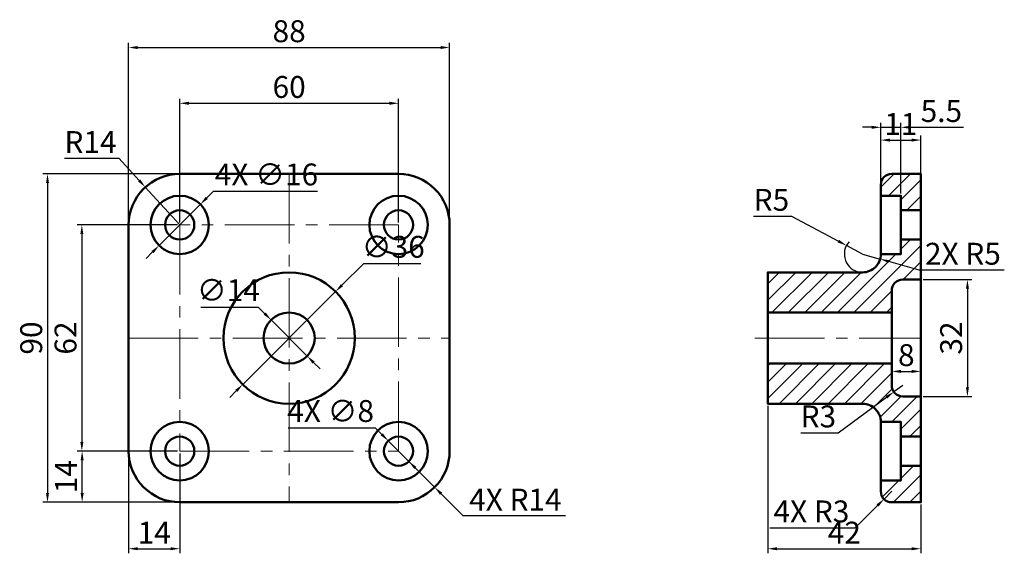
# Model space of a CAD drawing. Units: millimetres. Extents: x 7 to 277, y 39 to 185.
import ezdxf

# ---------------------------------------------------------------- set-up
doc = ezdxf.new("R2010")
doc.units = ezdxf.units.MM
doc.linetypes.add('CENTER2', pattern=[28.575, 19.05, -3.175, 3.175, -3.175])
for name, color, linetype, lineweight in [('M-CNTR', 4, 'CENTER2', 18), ('M-DIMS', 2, 'Continuous', 25), ('M-HATC', 8, 'Continuous', 18), ('M-OUTL', 7, 'Continuous', 50)]:
    doc.layers.add(name, color=color, linetype=linetype, lineweight=lineweight)
doc.styles.get("Standard").update_dxf_attribs({"font": 'arial.ttf'})
doc.dimstyles.new('ISO-25', dxfattribs={"dimtxt": 6, "dimasz": 2.5, "dimexe": 1.25, "dimexo": 0.625, "dimtad": 1, "dimtoh": 1, "dimdec": 0, "dimtxsty": 'Standard', "dimcen": 2.5, "dimadec": 0, "dimazin": 0, "dimtfac": 1, "dimtdec": 0, "dimtmove": 0, "dimatfit": 3, "dimfxl": 1, "dimarcsym": 0})

# ---------------------------------------------------------------- blocks, each defined once
blk = doc.blocks.new('*D1')
at = {"layer": 'Defpoints', "color": 0, "transparency": 16777216}
for p in [(233.41, 123.57), (237.82, 121.21)]:
    blk.add_point(p, dxfattribs=at)
at = {"layer": 'M-DIMS', "color": 0, "lineweight": -2, "transparency": 16777216}
for p, q in [((207.96, 131.63), (218.31, 131.63)), ((218.31, 131.63), (231.21, 124.75)), ((237.82, 121.21), (233.41, 123.57))]:
    blk.add_line(p, q, dxfattribs=at)
blk.add_arc((237.82, 121.21), 5, 137.5732, 262.838, dxfattribs=at)
at = {"layer": 'M-DIMS', "color": 0, "transparency": 16777216}
blk.add_solid([(231.4, 125.11), (231.01, 124.38), (233.41, 123.57)], dxfattribs=at)
at = {"layer": 'M-DIMS', "color": 0, "transparency": 16777216, "insert": (212.83, 135.31), "char_height": 6, "attachment_point": 5}
blk.add_mtext('R5', dxfattribs=at)
blk = doc.blocks.new('*D2')
at = {"layer": 'Defpoints', "color": 0, "transparency": 16777216}
for p in [(248.82, 85.21), (246.4, 83.44)]:
    blk.add_point(p, dxfattribs=at)
at = {"layer": 'M-DIMS', "color": 0, "lineweight": -2, "transparency": 16777216}
for p, q in [((248.82, 85.21), (246.4, 83.44)), ((231.16, 72.26), (244.39, 81.96)), ((220.86, 72.26), (231.16, 72.26))]:
    blk.add_line(p, q, dxfattribs=at)
at = {"layer": 'M-DIMS', "color": 0, "transparency": 16777216}
blk.add_solid([(244.14, 82.3), (244.63, 81.62), (246.4, 83.44)], dxfattribs=at)
at = {"layer": 'M-DIMS', "color": 0, "transparency": 16777216, "insert": (225.7, 75.95), "char_height": 6, "attachment_point": 5}
blk.add_mtext('R3', dxfattribs=at)
blk = doc.blocks.new('*D3')
at = {"layer": 'Defpoints', "color": 0, "transparency": 16777216}
for p in [(245.82, 91.21), (253.82, 91.21), (253.82, 89.06)]:
    blk.add_point(p, dxfattribs=at)
at = {"layer": 'M-DIMS', "color": 0, "lineweight": -2, "transparency": 16777216}
for p, q in [((245.82, 90.59), (245.82, 87.81)), ((253.82, 90.59), (253.82, 87.81)), ((248.32, 89.06), (251.32, 89.06))]:
    blk.add_line(p, q, dxfattribs=at)
at = {"layer": 'M-DIMS', "color": 0, "transparency": 16777216}
for points in [[(248.32, 89.48), (248.32, 88.65), (245.82, 89.06)], [(251.32, 89.48), (251.32, 88.65), (253.82, 89.06)]]:
    blk.add_solid(points, dxfattribs=at)
at = {"layer": 'M-DIMS', "color": 0, "transparency": 16777216, "insert": (249.82, 92.75), "char_height": 6, "attachment_point": 5}
blk.add_mtext('8', dxfattribs=at)
blk = doc.blocks.new('*D4')
at = {"layer": 'Defpoints', "color": 0, "transparency": 16777216}
for p in [(253.82, 152.47), (242.82, 137.21), (253.82, 137.21)]:
    blk.add_point(p, dxfattribs=at)
at = {"layer": 'M-DIMS', "color": 0, "lineweight": -2, "transparency": 16777216}
for p, q in [((242.82, 137.84), (242.82, 153.72)), ((245.32, 152.47), (251.32, 152.47)), ((253.82, 137.84), (253.82, 153.72))]:
    blk.add_line(p, q, dxfattribs=at)
at = {"layer": 'M-DIMS', "color": 0, "transparency": 16777216}
for points in [[(245.32, 152.88), (245.32, 152.05), (242.82, 152.47)], [(251.32, 152.88), (251.32, 152.05), (253.82, 152.47)]]:
    blk.add_solid(points, dxfattribs=at)
at = {"layer": 'M-DIMS', "color": 0, "transparency": 16777216, "insert": (248.32, 156.1), "char_height": 6, "attachment_point": 5}
blk.add_mtext('11', dxfattribs=at)
blk = doc.blocks.new('*D5')
at = {"layer": 'Defpoints', "color": 0, "transparency": 16777216}
for p in [(41.17, 139.56), (50.6, 129.21)]:
    blk.add_point(p, dxfattribs=at)
at = {"layer": 'M-DIMS', "color": 0, "lineweight": -2, "transparency": 16777216}
for p, q in [((18.98, 147.51), (33.91, 147.51)), ((33.91, 147.51), (39.48, 141.41)), ((50.6, 129.21), (41.17, 139.56))]:
    blk.add_line(p, q, dxfattribs=at)
at = {"layer": 'M-DIMS', "color": 0, "transparency": 16777216}
blk.add_solid([(39.79, 141.69), (39.17, 141.12), (41.17, 139.56)], dxfattribs=at)
at = {"layer": 'M-DIMS', "color": 0, "transparency": 16777216, "insert": (26.13, 151.15), "char_height": 6, "attachment_point": 5}
blk.add_mtext('R14', dxfattribs=at)
blk = doc.blocks.new('*D6')
at = {"layer": 'Defpoints', "color": 0, "transparency": 16777216}
for p in [(50.6, 129.21), (23.76, 67.21), (50.6, 67.21)]:
    blk.add_point(p, dxfattribs=at)
at = {"layer": 'M-DIMS', "color": 0, "lineweight": -2, "transparency": 16777216}
for p, q in [((49.97, 129.21), (22.51, 129.21)), ((23.76, 126.71), (23.76, 69.71)), ((49.97, 67.21), (22.51, 67.21))]:
    blk.add_line(p, q, dxfattribs=at)
at = {"layer": 'M-DIMS', "color": 0, "transparency": 16777216}
for points in [[(23.35, 126.71), (24.18, 126.71), (23.76, 129.21)], [(23.35, 69.71), (24.18, 69.71), (23.76, 67.21)]]:
    blk.add_solid(points, dxfattribs=at)
at = {"layer": 'M-DIMS', "color": 0, "transparency": 16777216, "insert": (20.07, 98.21), "char_height": 6, "attachment_point": 5, "rotation": 90}
blk.add_mtext('62', dxfattribs=at)
blk = doc.blocks.new('*D7')
at = {"layer": 'Defpoints', "color": 0, "transparency": 16777216}
for p in [(110.6, 162.55), (50.6, 129.21), (110.6, 129.21)]:
    blk.add_point(p, dxfattribs=at)
at = {"layer": 'M-DIMS', "color": 0, "lineweight": -2, "transparency": 16777216}
for p, q in [((50.6, 129.84), (50.6, 163.8)), ((53.1, 162.55), (108.1, 162.55)), ((110.6, 129.84), (110.6, 163.8))]:
    blk.add_line(p, q, dxfattribs=at)
at = {"layer": 'M-DIMS', "color": 0, "transparency": 16777216}
for points in [[(53.1, 162.97), (53.1, 162.13), (50.6, 162.55)], [(108.1, 162.97), (108.1, 162.13), (110.6, 162.55)]]:
    blk.add_solid(points, dxfattribs=at)
at = {"layer": 'M-DIMS', "color": 0, "transparency": 16777216, "insert": (80.6, 166.24), "char_height": 6, "attachment_point": 5}
blk.add_mtext('60', dxfattribs=at)
blk = doc.blocks.new('*D8')
at = {"layer": 'Defpoints', "color": 0, "transparency": 16777216}
for p in [(124.6, 177.83), (36.6, 109.01), (124.6, 109.01)]:
    blk.add_point(p, dxfattribs=at)
at = {"layer": 'M-DIMS', "color": 0, "lineweight": -2, "transparency": 16777216}
for p, q in [((36.6, 109.64), (36.6, 179.08)), ((124.6, 109.64), (124.6, 179.08)), ((39.1, 177.83), (122.1, 177.83))]:
    blk.add_line(p, q, dxfattribs=at)
at = {"layer": 'M-DIMS', "color": 0, "transparency": 16777216}
for points in [[(39.1, 178.25), (39.1, 177.41), (36.6, 177.83)], [(122.1, 178.25), (122.1, 177.41), (124.6, 177.83)]]:
    blk.add_solid(points, dxfattribs=at)
at = {"layer": 'M-DIMS', "color": 0, "transparency": 16777216, "insert": (80.6, 181.52), "char_height": 6, "attachment_point": 5}
blk.add_mtext('88', dxfattribs=at)
blk = doc.blocks.new('*D9')
at = {"layer": 'Defpoints', "color": 0, "transparency": 16777216}
for p in [(62.7, 143.21), (14.35, 53.21), (62.7, 53.21)]:
    blk.add_point(p, dxfattribs=at)
at = {"layer": 'M-DIMS', "color": 0, "lineweight": -2, "transparency": 16777216}
for p, q in [((62.07, 143.21), (13.1, 143.21)), ((14.35, 140.71), (14.35, 55.71)), ((62.07, 53.21), (13.1, 53.21))]:
    blk.add_line(p, q, dxfattribs=at)
at = {"layer": 'M-DIMS', "color": 0, "transparency": 16777216}
for points in [[(13.93, 140.71), (14.76, 140.71), (14.35, 143.21)], [(13.93, 55.71), (14.76, 55.71), (14.35, 53.21)]]:
    blk.add_solid(points, dxfattribs=at)
at = {"layer": 'M-DIMS', "color": 0, "transparency": 16777216, "insert": (10.66, 98.21), "char_height": 6, "attachment_point": 5, "rotation": 90}
blk.add_mtext('90', dxfattribs=at)
blk = doc.blocks.new('HOLE-CBORE-D8-D16')
for radius in [8, 4]:
    blk.add_circle((8, 8), radius)
blk = doc.blocks.new('*D11')
at = {"layer": 'Defpoints', "color": 0, "transparency": 16777216}
for p in [(211.82, 80.21), (253.82, 53.21), (253.82, 40.46)]:
    blk.add_point(p, dxfattribs=at)
at = {"layer": 'M-DIMS', "color": 0, "lineweight": -2, "transparency": 16777216}
for p, q in [((211.82, 79.59), (211.82, 39.21)), ((253.82, 52.59), (253.82, 39.21)), ((214.32, 40.46), (251.32, 40.46))]:
    blk.add_line(p, q, dxfattribs=at)
at = {"layer": 'M-DIMS', "color": 0, "transparency": 16777216}
for points in [[(214.32, 40.88), (214.32, 40.05), (211.82, 40.46)], [(251.32, 40.88), (251.32, 40.05), (253.82, 40.46)]]:
    blk.add_solid(points, dxfattribs=at)
at = {"layer": 'M-DIMS', "color": 0, "transparency": 16777216, "insert": (232.82, 44.1), "char_height": 6, "attachment_point": 5}
blk.add_mtext('42', dxfattribs=at)
blk = doc.blocks.new('*D12')
at = {"layer": 'Defpoints', "color": 0, "transparency": 16777216}
for p in [(253.82, 114.21), (253.82, 82.21), (266.57, 82.21)]:
    blk.add_point(p, dxfattribs=at)
at = {"layer": 'M-DIMS', "color": 0, "lineweight": -2, "transparency": 16777216}
for p, q in [((254.45, 114.21), (267.82, 114.21)), ((266.57, 111.71), (266.57, 84.71)), ((254.45, 82.21), (267.82, 82.21))]:
    blk.add_line(p, q, dxfattribs=at)
at = {"layer": 'M-DIMS', "color": 0, "transparency": 16777216}
for points in [[(266.16, 111.71), (266.99, 111.71), (266.57, 114.21)], [(266.16, 84.71), (266.99, 84.71), (266.57, 82.21)]]:
    blk.add_solid(points, dxfattribs=at)
at = {"layer": 'M-DIMS', "color": 0, "transparency": 16777216, "insert": (262.88, 98.21), "char_height": 6, "attachment_point": 5, "rotation": 90}
blk.add_mtext('32', dxfattribs=at)
blk = doc.blocks.new('*D13')
at = {"layer": 'Defpoints', "color": 0, "transparency": 16777216}
for p in [(248.32, 155.96), (242.82, 137.21), (248.32, 137.21)]:
    blk.add_point(p, dxfattribs=at)
at = {"layer": 'M-DIMS', "color": 0, "lineweight": -2, "transparency": 16777216}
for p, q in [((242.82, 137.84), (242.82, 157.21)), ((248.32, 137.84), (248.32, 157.21)), ((240.32, 155.96), (237.82, 155.96)), ((242.82, 155.96), (248.32, 155.96)), ((250.82, 155.96), (265.54, 155.96))]:
    blk.add_line(p, q, dxfattribs=at)
at = {"layer": 'M-DIMS', "color": 0, "transparency": 16777216}
for points in [[(240.32, 156.38), (240.32, 155.55), (242.82, 155.96)], [(250.82, 156.38), (250.82, 155.55), (248.32, 155.96)]]:
    blk.add_solid(points, dxfattribs=at)
at = {"layer": 'M-DIMS', "color": 0, "transparency": 16777216, "insert": (259.43, 159.64), "char_height": 6, "attachment_point": 5}
blk.add_mtext('5.5', dxfattribs=at)
blk = doc.blocks.new('*D14')
at = {"layer": 'Defpoints', "color": 0, "transparency": 16777216}
for p in [(36.6, 67.21), (50.6, 67.21), (50.6, 40.46)]:
    blk.add_point(p, dxfattribs=at)
at = {"layer": 'M-DIMS', "color": 0, "lineweight": -2, "transparency": 16777216}
for p, q in [((36.6, 66.59), (36.6, 39.21)), ((50.6, 66.59), (50.6, 39.21)), ((39.1, 40.46), (48.1, 40.46))]:
    blk.add_line(p, q, dxfattribs=at)
at = {"layer": 'M-DIMS', "color": 0, "transparency": 16777216}
for points in [[(39.1, 40.88), (39.1, 40.05), (36.6, 40.46)], [(48.1, 40.88), (48.1, 40.05), (50.6, 40.46)]]:
    blk.add_solid(points, dxfattribs=at)
at = {"layer": 'M-DIMS', "color": 0, "transparency": 16777216, "insert": (43.6, 44.1), "char_height": 6, "attachment_point": 5}
blk.add_mtext('14', dxfattribs=at)
blk = doc.blocks.new('*D15')
at = {"layer": 'Defpoints', "color": 0, "transparency": 16777216}
for p in [(23.85, 67.21), (50.6, 67.21), (50.6, 53.21)]:
    blk.add_point(p, dxfattribs=at)
at = {"layer": 'M-DIMS', "color": 0, "lineweight": -2, "transparency": 16777216}
for p, q in [((49.97, 67.21), (22.6, 67.21)), ((23.85, 55.71), (23.85, 64.71)), ((49.97, 53.21), (22.6, 53.21))]:
    blk.add_line(p, q, dxfattribs=at)
at = {"layer": 'M-DIMS', "color": 0, "transparency": 16777216}
for points in [[(23.43, 64.71), (24.26, 64.71), (23.85, 67.21)], [(23.43, 55.71), (24.26, 55.71), (23.85, 53.21)]]:
    blk.add_solid(points, dxfattribs=at)
at = {"layer": 'M-DIMS', "color": 0, "transparency": 16777216, "insert": (20.21, 60.21), "char_height": 6, "attachment_point": 5, "rotation": 90}
blk.add_mtext('14', dxfattribs=at)
blk = doc.blocks.new('*D16')
at = {"layer": 'Defpoints', "color": 0, "transparency": 16777216}
for p in [(110.6, 67.21), (120.5, 57.31)]:
    blk.add_point(p, dxfattribs=at)
at = {"layer": 'M-DIMS', "color": 0, "lineweight": -2, "transparency": 16777216}
for p, q in [((110.6, 67.21), (120.5, 57.31)), ((128.3, 49.52), (122.27, 55.55)), ((156.37, 49.52), (128.3, 49.52))]:
    blk.add_line(p, q, dxfattribs=at)
at = {"layer": 'M-DIMS', "color": 0, "transparency": 16777216}
blk.add_solid([(122.56, 55.84), (121.97, 55.25), (120.5, 57.31)], dxfattribs=at)
at = {"layer": 'M-DIMS', "color": 0, "transparency": 16777216, "insert": (142.64, 53.16), "char_height": 6, "attachment_point": 5}
blk.add_mtext('4X R14', dxfattribs=at)
blk = doc.blocks.new('*D17')
at = {"layer": 'Defpoints', "color": 0, "transparency": 16777216}
for p in [(56.26, 134.87), (44.94, 123.56)]:
    blk.add_point(p, dxfattribs=at)
at = {"layer": 'M-DIMS', "color": 0, "lineweight": -2, "transparency": 16777216}
for p, q in [((59.79, 138.41), (58.02, 136.64)), ((88.35, 138.41), (59.79, 138.41)), ((44.94, 123.56), (56.26, 134.87)), ((43.17, 121.79), (41.41, 120.02))]:
    blk.add_line(p, q, dxfattribs=at)
at = {"layer": 'M-DIMS', "color": 0, "transparency": 16777216}
for points in [[(57.73, 136.93), (58.32, 136.34), (56.26, 134.87)], [(42.88, 122.08), (43.47, 121.49), (44.94, 123.56)]]:
    blk.add_solid(points, dxfattribs=at)
at = {"layer": 'M-DIMS', "color": 0, "transparency": 16777216, "insert": (74.38, 142.26), "char_height": 6, "attachment_point": 5}
blk.add_mtext('4X ∅16', dxfattribs=at)
blk = doc.blocks.new('*D18')
at = {"layer": 'Defpoints', "color": 0, "transparency": 16777216}
for p in [(107.77, 70.04), (113.43, 64.38)]:
    blk.add_point(p, dxfattribs=at)
at = {"layer": 'M-DIMS', "color": 0, "lineweight": -2, "transparency": 16777216}
for p, q in [((80.32, 73.58), (104.23, 73.58)), ((104.23, 73.58), (106, 71.81)), ((113.43, 64.38), (107.77, 70.04)), ((115.19, 62.62), (116.96, 60.85))]:
    blk.add_line(p, q, dxfattribs=at)
at = {"layer": 'M-DIMS', "color": 0, "transparency": 16777216}
for points in [[(106.3, 72.1), (105.71, 71.52), (107.77, 70.04)], [(115.49, 62.91), (114.9, 62.32), (113.43, 64.38)]]:
    blk.add_solid(points, dxfattribs=at)
at = {"layer": 'M-DIMS', "color": 0, "transparency": 16777216, "insert": (91.97, 77.43), "char_height": 6, "attachment_point": 5}
blk.add_mtext('4X ∅8', dxfattribs=at)
blk = doc.blocks.new('*D19')
at = {"layer": 'Defpoints', "color": 0, "transparency": 16777216}
for p in [(93.33, 110.94), (67.87, 85.49)]:
    blk.add_point(p, dxfattribs=at)
at = {"layer": 'M-DIMS', "color": 0, "lineweight": -2, "transparency": 16777216}
for p, q in [((100.96, 118.58), (95.09, 112.71)), ((116.71, 118.58), (100.96, 118.58)), ((67.87, 85.49), (93.33, 110.94)), ((66.1, 83.72), (64.33, 81.95))]:
    blk.add_line(p, q, dxfattribs=at)
at = {"layer": 'M-DIMS', "color": 0, "transparency": 16777216}
for points in [[(94.8, 113), (95.39, 112.41), (93.33, 110.94)], [(65.81, 84.01), (66.4, 83.42), (67.87, 85.49)]]:
    blk.add_solid(points, dxfattribs=at)
at = {"layer": 'M-DIMS', "color": 0, "transparency": 16777216, "insert": (109.15, 122.43), "char_height": 6, "attachment_point": 5}
blk.add_mtext('∅36', dxfattribs=at)
blk = doc.blocks.new('*D20')
at = {"layer": 'Defpoints', "color": 0, "transparency": 16777216}
for p in [(75.65, 103.16), (85.55, 93.26)]:
    blk.add_point(p, dxfattribs=at)
at = {"layer": 'M-DIMS', "color": 0, "lineweight": -2, "transparency": 16777216}
for p, q in [((56.39, 106.7), (72.11, 106.7)), ((72.11, 106.7), (73.88, 104.93)), ((85.55, 93.26), (75.65, 103.16)), ((87.32, 91.5), (89.08, 89.73))]:
    blk.add_line(p, q, dxfattribs=at)
at = {"layer": 'M-DIMS', "color": 0, "transparency": 16777216}
for points in [[(74.17, 105.23), (73.59, 104.64), (75.65, 103.16)], [(87.61, 91.79), (87.02, 91.2), (85.55, 93.26)]]:
    blk.add_solid(points, dxfattribs=at)
at = {"layer": 'M-DIMS', "color": 0, "transparency": 16777216, "insert": (63.94, 110.55), "char_height": 6, "attachment_point": 5}
blk.add_mtext('∅14', dxfattribs=at)
blk = doc.blocks.new('*D21')
at = {"layer": 'Defpoints', "color": 0, "transparency": 16777216}
for p in [(237.82, 121.21), (242.63, 119.86)]:
    blk.add_point(p, dxfattribs=at)
at = {"layer": 'M-DIMS', "color": 0, "lineweight": -2, "transparency": 16777216}
for p, q in [((237.82, 121.21), (242.63, 119.86)), ((253.35, 116.84), (245.04, 119.18)), ((276.69, 116.84), (253.35, 116.84))]:
    blk.add_line(p, q, dxfattribs=at)
at = {"layer": 'M-DIMS', "color": 0, "transparency": 16777216}
blk.add_solid([(245.15, 119.58), (244.93, 118.78), (242.63, 119.86)], dxfattribs=at)
at = {"layer": 'M-DIMS', "color": 0, "transparency": 16777216, "insert": (265.33, 120.53), "char_height": 6, "attachment_point": 5}
blk.add_mtext('2X R5', dxfattribs=at)
blk = doc.blocks.new('*D22')
at = {"layer": 'Defpoints', "color": 0, "transparency": 16777216}
for p in [(243.7, 54.09), (245.82, 56.21)]:
    blk.add_point(p, dxfattribs=at)
at = {"layer": 'M-DIMS', "color": 0, "lineweight": -2, "transparency": 16777216}
for p, q in [((245.82, 56.21), (243.7, 54.09)), ((235.83, 46.22), (241.93, 52.32)), ((212.39, 46.22), (235.83, 46.22))]:
    blk.add_line(p, q, dxfattribs=at)
at = {"layer": 'M-DIMS', "color": 0, "transparency": 16777216}
blk.add_solid([(241.64, 52.62), (242.23, 52.03), (243.7, 54.09)], dxfattribs=at)
at = {"layer": 'M-DIMS', "color": 0, "transparency": 16777216, "insert": (223.8, 49.91), "char_height": 6, "attachment_point": 5}
blk.add_mtext('4X R3', dxfattribs=at)

msp = doc.modelspace()

# ---------------------------------------------------------------- hatches: boundary and pattern name
at = {"layer": 'M-HATC'}
h = msp.add_hatch(dxfattribs=at)
h.set_pattern_fill('ANSI31', color=256)
h.paths.add_polyline_path([(253.82, 143.21), (245.82, 143.21, 0.414214), (242.82, 140.21), (242.82, 137.21), (248.32, 137.21), (248.32, 133.21), (253.82, 133.21)])
h.paths.add_polyline_path([(248.82, 114.21), (253.82, 114.21), (253.82, 125.21), (248.32, 125.21), (248.32, 121.21), (242.82, 121.21, -0.414214), (237.82, 116.21), (211.82, 116.21), (211.82, 105.21), (245.82, 105.21), (245.82, 111.21, -0.414214)])
h.paths.add_polyline_path([(245.82, 91.21), (211.82, 91.21), (211.82, 80.21), (237.82, 80.21, -0.414214), (242.82, 75.21), (248.32, 75.21), (248.32, 71.21), (253.82, 71.21), (253.82, 82.21), (248.82, 82.21, -0.414214), (245.82, 85.21)])
h.paths.add_polyline_path([(253.82, 63.21), (248.32, 63.21), (248.32, 59.21), (242.82, 59.21), (242.82, 56.21, 0.414214), (245.82, 53.21), (253.82, 53.21)])

# ---------------------------------------------------------------- linework, layer by layer
at = {"layer": 'M-CNTR'}
for p, q in [((80.6, 143.21), (80.6, 53.21)), ((36.6, 98.21), (124.6, 98.21)), ((208.32, 98.21), (253.82, 98.21))]:
    msp.add_line(p, q, dxfattribs=at)
msp.add_lwpolyline([(110.6, 67.21), (110.6, 129.21), (50.6, 129.21), (50.6, 67.21)], close=True, dxfattribs=at)
at = {"layer": 'M-OUTL'}
for p, q in [((211.82, 105.21), (245.82, 105.21)), ((211.82, 91.21), (245.82, 91.21)), ((248.32, 71.21), (253.82, 71.21)), ((248.32, 63.21), (253.82, 63.21))]:
    msp.add_line(p, q, dxfattribs=at)
msp.add_lwpolyline([(36.6, 67.21, 0.414214), (50.6, 53.21), (110.6, 53.21, 0.414214), (124.6, 67.21), (124.6, 129.21, 0.414214), (110.6, 143.21), (50.6, 143.21, 0.414214), (36.6, 129.21)], format="xyb", close=True, dxfattribs=at)
for points in [[(242.82, 75.21), (242.82, 56.21, 0.414214), (245.82, 53.21), (253.82, 53.21), (253.82, 143.21), (245.82, 143.21, 0.414214), (242.82, 140.21), (242.82, 121.21, -0.414214), (237.82, 116.21), (211.82, 116.21), (211.82, 80.21), (237.82, 80.21, -0.414214), (242.82, 75.21), (248.32, 75.21), (248.32, 59.21), (242.82, 59.21)], [(253.82, 114.21), (248.82, 114.21, 0.414214), (245.82, 111.21), (245.82, 85.21, 0.414214), (248.82, 82.21), (253.82, 82.21)]]:
    msp.add_lwpolyline(points, format="xyb", dxfattribs=at)
for points in [[(242.82, 137.21), (248.32, 137.21), (248.32, 121.21), (242.82, 121.21), (248.32, 121.21), (248.32, 137.21)], [(248.32, 133.21), (253.82, 133.21)], [(248.32, 125.21), (253.82, 125.21)]]:
    msp.add_lwpolyline(points, close=True, dxfattribs=at)
for radius in [18, 7]:
    msp.add_circle((80.6, 98.21), radius, dxfattribs=at)

# ---------------------------------------------------------------- block references
for p in [(42.6, 121.21), (102.6, 121.21), (42.6, 59.21), (102.6, 59.21)]:
    msp.add_blockref('HOLE-CBORE-D8-D16', p, dxfattribs=at)

# ---------------------------------------------------------------- dimensions: what is measured, and where the dimension line sits
at = {"layer": 'M-DIMS'}
for base, p1, p2, override, picture, middle in [((124.6, 177.83), (36.6, 109.01), (124.6, 109.01), {"dimclrd": 0, "dimclre": 0, "dimclrt": 0}, '*D8', (80.6, 181.52)), ((110.6, 162.55), (50.6, 129.21), (110.6, 129.21), {"dimclrd": 0, "dimclre": 0, "dimclrt": 0}, '*D7', (80.6, 166.24)), ((248.32, 155.96), (242.82, 137.21), (248.32, 137.21), {"dimdec": 1, "dimlfac": 1, "dimrnd": 0, "dimzin": 0, "dimdsep": 46, "dimlunit": 2}, '*D13', (259.43, 159.64)), ((253.82, 152.47), (242.82, 137.21), (253.82, 137.21), {"dimclrd": 0, "dimclre": 0, "dimclrt": 0}, '*D4', (248.32, 156.1)), ((253.82, 89.06), (245.82, 91.21), (253.82, 91.21), {"dimclrd": 0, "dimclre": 0, "dimclrt": 0}, '*D3', (249.82, 92.75)), ((253.82, 40.46), (211.82, 80.21), (253.82, 53.21), {"dimdec": 0, "dimlfac": 1, "dimrnd": 0, "dimzin": 0, "dimdsep": 46, "dimlunit": 2}, '*D11', (232.82, 44.1)), ((50.6, 40.46), (36.6, 67.21), (50.6, 67.21), {"dimdec": 0, "dimlfac": 1, "dimrnd": 0, "dimzin": 0, "dimdsep": 46, "dimlunit": 2}, '*D14', (43.6, 44.1))]:
    dim = msp.add_linear_dim(base=base, p1=p1, p2=p2, dimstyle='ISO-25', override=override, dxfattribs=at)
    dim.commit()
    dim.dimension.update_dxf_attribs({"geometry": picture, "text_midpoint": middle})
for center, mpoint, picture, middle in [((50.6, 129.21), (41.17, 139.56), '*D5', (26.13, 147.51)), ((237.82, 121.21), (233.41, 123.57), '*D1', (212.83, 131.63)), ((248.82, 85.21), (246.4, 83.44), '*D2', (225.7, 72.26))]:
    dim = msp.add_radius_dim(center=center, mpoint=mpoint, dimstyle='ISO-25', override={"dimclrd": 0, "dimclre": 0, "dimclrt": 0}, dxfattribs=at)
    dim.commit()
    dim.dimension.update_dxf_attribs({"geometry": picture, "text_midpoint": middle, "dimtype": 164})
for p1, p2, picture, middle in [((44.94, 123.56), (56.26, 134.87), '*D17', (74.38, 138.41)), ((113.43, 64.38), (107.77, 70.04), '*D18', (91.97, 73.58))]:
    dim = msp.add_diameter_dim_2p(p1=p1, p2=p2, text='4X <>', dimstyle='ISO-25', override={"dimdec": 0, "dimlfac": 1, "dimrnd": 0, "dimzin": 0, "dimdsep": 46, "dimlunit": 2}, dxfattribs=at)
    dim.commit()
    dim.dimension.update_dxf_attribs({"geometry": picture, "text_midpoint": middle, "dimtype": 163})
for base, p1, p2, override, picture, middle in [((14.35, 53.21), (62.7, 143.21), (62.7, 53.21), {"dimclrd": 0, "dimclre": 0, "dimclrt": 0}, '*D9', (10.66, 98.21)), ((23.76, 67.21), (50.6, 129.21), (50.6, 67.21), {"dimclrd": 0, "dimclre": 0, "dimclrt": 0}, '*D6', (20.07, 98.21)), ((266.57, 82.21), (253.82, 114.21), (253.82, 82.21), {"dimdec": 0, "dimlfac": 1, "dimrnd": 0, "dimzin": 0, "dimdsep": 46, "dimlunit": 2}, '*D12', (262.88, 98.21)), ((23.85, 67.21), (50.6, 53.21), (50.6, 67.21), {"dimdec": 0, "dimlfac": 1, "dimrnd": 0, "dimzin": 0, "dimdsep": 46, "dimlunit": 2}, '*D15', (20.21, 60.21))]:
    dim = msp.add_linear_dim(base=base, p1=p1, p2=p2, angle=90, dimstyle='ISO-25', override=override, dxfattribs=at)
    dim.commit()
    dim.dimension.update_dxf_attribs({"geometry": picture, "text_midpoint": middle})
for center, mpoint, text, picture, middle in [((237.82, 121.21), (242.63, 119.86), '2X <>', '*D21', (265.33, 120.53)), ((110.6, 67.21), (120.5, 57.31), '4X <>', '*D16', (142.64, 53.16)), ((245.82, 56.21), (243.7, 54.09), '4X <>', '*D22', (223.8, 49.91))]:
    dim = msp.add_radius_dim(center=center, mpoint=mpoint, text=text, dimstyle='ISO-25', override={"dimdec": 0, "dimlfac": 1, "dimrnd": 0, "dimzin": 0, "dimdsep": 46, "dimlunit": 2}, dxfattribs=at)
    dim.commit()
    dim.dimension.update_dxf_attribs({"geometry": picture, "text_midpoint": middle})
for p1, p2, picture, middle in [((67.87, 85.49), (93.33, 110.94), '*D19', (109.15, 118.58)), ((85.55, 93.26), (75.65, 103.16), '*D20', (63.94, 106.7))]:
    dim = msp.add_diameter_dim_2p(p1=p1, p2=p2, dimstyle='ISO-25', override={"dimdec": 0, "dimlfac": 1, "dimrnd": 0, "dimzin": 0, "dimdsep": 46, "dimlunit": 2}, dxfattribs=at)
    dim.commit()
    dim.dimension.update_dxf_attribs({"geometry": picture, "text_midpoint": middle, "dimtype": 163})

doc.saveas('drawing.dxf')
